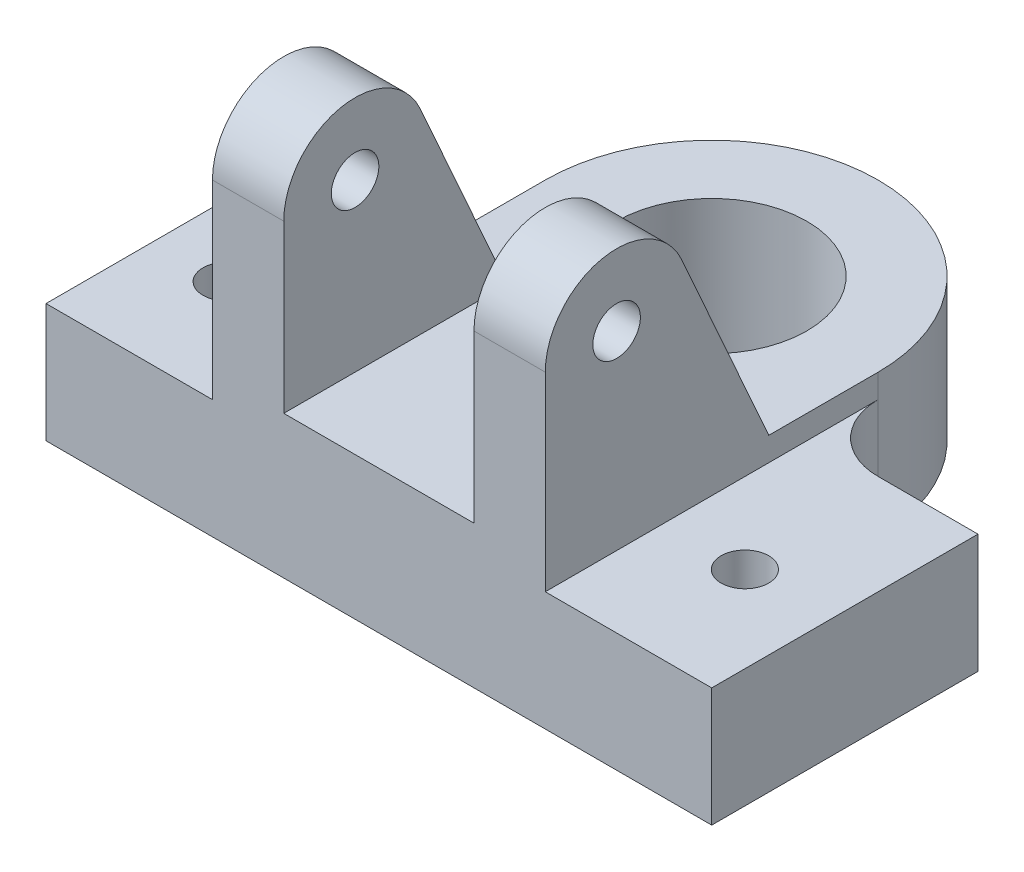
ISO-10303-21;
HEADER;
FILE_DESCRIPTION(('STEP AP214'),'2;1');
FILE_NAME('part.step','',(''),(''),'','','');
FILE_SCHEMA(('AUTOMOTIVE_DESIGN { 1 0 10303 214 1 1 1 1 }'));
ENDSEC;
DATA;
#1=APPLICATION_CONTEXT('core data for automotive mechanical design processes');
#2=APPLICATION_PROTOCOL_DEFINITION('international standard','automotive_design',2000,#1);
#3=PRODUCT_CONTEXT('',#1,'mechanical');
#4=PRODUCT('Part','Part','',(#3));
#5=PRODUCT_RELATED_PRODUCT_CATEGORY('part','',(#4));
#6=PRODUCT_DEFINITION_FORMATION('','',#4);
#7=PRODUCT_DEFINITION_CONTEXT('part definition',#1,'design');
#8=PRODUCT_DEFINITION('design','',#6,#7);
#9=PRODUCT_DEFINITION_SHAPE('','',#8);
#10=(LENGTH_UNIT() NAMED_UNIT(*) SI_UNIT(.MILLI.,.METRE.));
#11=(NAMED_UNIT(*) PLANE_ANGLE_UNIT() SI_UNIT($,.RADIAN.));
#12=(NAMED_UNIT(*) SI_UNIT($,.STERADIAN.) SOLID_ANGLE_UNIT());
#13=UNCERTAINTY_MEASURE_WITH_UNIT(LENGTH_MEASURE(1.E-05),#10,'distance_accuracy_value','');
#14=(GEOMETRIC_REPRESENTATION_CONTEXT(3) GLOBAL_UNCERTAINTY_ASSIGNED_CONTEXT((#13)) GLOBAL_UNIT_ASSIGNED_CONTEXT((#10,
#11,#12)) REPRESENTATION_CONTEXT('',''));
#15=CARTESIAN_POINT('',(0.,0.,0.));
#16=DIRECTION('',(0.,0.,1.));
#17=DIRECTION('',(1.,0.,0.));
#18=AXIS2_PLACEMENT_3D('',#15,#16,#17);
#19=CARTESIAN_POINT('',(-70.,25.,31.7302464178724));
#20=DIRECTION('',(0.,0.,-1.));
#21=DIRECTION('',(-1.,0.,0.));
#22=AXIS2_PLACEMENT_3D('',#19,#20,#21);
#23=PLANE('',#22);
#24=DIRECTION('',(0.,-1.,0.));
#25=VECTOR('',#24,1.);
#26=CARTESIAN_POINT('',(-20.,237.,31.7302464178724));
#27=LINE('',#26,#25);
#28=CARTESIAN_POINT('',(-20.,65.0000000000001,31.7302464178724));
#29=VERTEX_POINT('',#28);
#30=CARTESIAN_POINT('',(-20.,30.,31.7302464178724));
#31=VERTEX_POINT('',#30);
#32=EDGE_CURVE('E167',#29,#31,#27,.T.);
#33=ORIENTED_EDGE('',*,*,#32,.F.);
#34=DIRECTION('',(1.,0.,0.));
#35=VECTOR('',#34,1.);
#36=CARTESIAN_POINT('',(-35.,65.,31.7302464178724));
#37=LINE('',#36,#35);
#38=CARTESIAN_POINT('',(-35.,65.,31.7302464178724));
#39=VERTEX_POINT('',#38);
#40=EDGE_CURVE('E192',#39,#29,#37,.T.);
#41=ORIENTED_EDGE('',*,*,#40,.F.);
#42=DIRECTION('',(0.,-1.,0.));
#43=VECTOR('',#42,1.);
#44=CARTESIAN_POINT('',(-35.,30.,31.7302464178724));
#45=LINE('',#44,#43);
#46=CARTESIAN_POINT('',(-35.,25.,31.7302464178724));
#47=VERTEX_POINT('',#46);
#48=EDGE_CURVE('E235',#39,#47,#45,.T.);
#49=ORIENTED_EDGE('',*,*,#48,.T.);
#50=DIRECTION('',(1.,0.,0.));
#51=VECTOR('',#50,1.);
#52=CARTESIAN_POINT('',(-70.,25.,31.7302464178724));
#53=LINE('',#52,#51);
#54=CARTESIAN_POINT('',(-70.,25.,31.7302464178724));
#55=VERTEX_POINT('',#54);
#56=EDGE_CURVE('E274',#55,#47,#53,.T.);
#57=ORIENTED_EDGE('',*,*,#56,.F.);
#58=DIRECTION('',(0.,-1.,0.));
#59=VECTOR('',#58,1.);
#60=CARTESIAN_POINT('',(-70.,25.,31.7302464178724));
#61=LINE('',#60,#59);
#62=CARTESIAN_POINT('',(-70.,0.,31.7302464178724));
#63=VERTEX_POINT('',#62);
#64=EDGE_CURVE('E283',#55,#63,#61,.T.);
#65=ORIENTED_EDGE('',*,*,#64,.T.);
#66=DIRECTION('',(1.,0.,0.));
#67=VECTOR('',#66,1.);
#68=CARTESIAN_POINT('',(-70.,0.,31.7302464178724));
#69=LINE('',#68,#67);
#70=CARTESIAN_POINT('',(70.,0.,31.7302464178724));
#71=VERTEX_POINT('',#70);
#72=EDGE_CURVE('E280',#63,#71,#69,.T.);
#73=ORIENTED_EDGE('',*,*,#72,.T.);
#74=DIRECTION('',(0.,-1.,0.));
#75=VECTOR('',#74,1.);
#76=CARTESIAN_POINT('',(70.,25.,31.7302464178724));
#77=LINE('',#76,#75);
#78=CARTESIAN_POINT('',(70.,25.,31.7302464178724));
#79=VERTEX_POINT('',#78);
#80=EDGE_CURVE('E279',#79,#71,#77,.T.);
#81=ORIENTED_EDGE('',*,*,#80,.F.);
#82=CARTESIAN_POINT('',(35.,25.,31.7302464178724));
#83=VERTEX_POINT('',#82);
#84=EDGE_CURVE('E271',#83,#79,#53,.T.);
#85=ORIENTED_EDGE('',*,*,#84,.F.);
#86=DIRECTION('',(0.,-1.,0.));
#87=VECTOR('',#86,1.);
#88=CARTESIAN_POINT('',(35.,30.,31.7302464178724));
#89=LINE('',#88,#87);
#90=CARTESIAN_POINT('',(35.,65.,31.7302464178724));
#91=VERTEX_POINT('',#90);
#92=EDGE_CURVE('E230',#91,#83,#89,.T.);
#93=ORIENTED_EDGE('',*,*,#92,.F.);
#94=CARTESIAN_POINT('',(20.,65.,31.7302464178724));
#95=VERTEX_POINT('',#94);
#96=EDGE_CURVE('E204',#95,#91,#37,.T.);
#97=ORIENTED_EDGE('',*,*,#96,.F.);
#98=DIRECTION('',(0.,-1.,0.));
#99=VECTOR('',#98,1.);
#100=CARTESIAN_POINT('',(20.,237.,31.7302464178725));
#101=LINE('',#100,#99);
#102=CARTESIAN_POINT('',(20.,30.,31.7302464178725));
#103=VERTEX_POINT('',#102);
#104=EDGE_CURVE('E56',#95,#103,#101,.T.);
#105=ORIENTED_EDGE('',*,*,#104,.T.);
#106=DIRECTION('',(1.,0.,0.));
#107=VECTOR('',#106,1.);
#108=CARTESIAN_POINT('',(-20.,30.,31.7302464178724));
#109=LINE('',#108,#107);
#110=EDGE_CURVE('E173',#31,#103,#109,.T.);
#111=ORIENTED_EDGE('',*,*,#110,.F.);
#112=EDGE_LOOP('',(#33,#41,#49,#57,#65,#73,#81,#85,#93,#97,#105,#111));
#113=FACE_BOUND('',#112,.T.);
#114=ADVANCED_FACE('F43',(#113),#23,.F.);
#115=CARTESIAN_POINT('',(-35.,10.635177862415,-23.8903273022607));
#116=DIRECTION('',(0.,0.406689373293844,-0.913566502040142));
#117=DIRECTION('',(0.,0.913566502040142,0.406689373293844));
#118=AXIS2_PLACEMENT_3D('',#115,#116,#117);
#119=PLANE('',#118);
#120=DIRECTION('',(1.,0.,0.));
#121=VECTOR('',#120,1.);
#122=CARTESIAN_POINT('',(-35.,71.1003405994077,3.02674888727032));
#123=LINE('',#122,#121);
#124=CARTESIAN_POINT('',(-35.,71.1003405994077,3.02674888727032));
#125=VERTEX_POINT('',#124);
#126=CARTESIAN_POINT('',(-20.,71.1003405994077,3.02674888727032));
#127=VERTEX_POINT('',#126);
#128=EDGE_CURVE('E185',#125,#127,#123,.T.);
#129=ORIENTED_EDGE('',*,*,#128,.T.);
#130=DIRECTION('',(0.,-0.913566502040142,-0.406689373293844));
#131=VECTOR('',#130,1.);
#132=CARTESIAN_POINT('',(-20.,10.635177862415,-23.8903273022607));
#133=LINE('',#132,#131);
#134=CARTESIAN_POINT('',(-20.,30.,-15.2697535821276));
#135=VERTEX_POINT('',#134);
#136=EDGE_CURVE('E166',#127,#135,#133,.T.);
#137=ORIENTED_EDGE('',*,*,#136,.T.);
#138=DIRECTION('',(1.,0.,0.));
#139=VECTOR('',#138,1.);
#140=CARTESIAN_POINT('',(-35.,30.,-15.2697535821276));
#141=LINE('',#140,#139);
#142=CARTESIAN_POINT('',(-35.,30.,-15.2697535821276));
#143=VERTEX_POINT('',#142);
#144=EDGE_CURVE('E179',#143,#135,#141,.T.);
#145=ORIENTED_EDGE('',*,*,#144,.F.);
#146=DIRECTION('',(0.,0.913566502040142,0.406689373293844));
#147=VECTOR('',#146,1.);
#148=CARTESIAN_POINT('',(-35.,10.635177862415,-23.8903273022607));
#149=LINE('',#148,#147);
#150=EDGE_CURVE('E319',#143,#125,#149,.T.);
#151=ORIENTED_EDGE('',*,*,#150,.T.);
#152=EDGE_LOOP('',(#129,#137,#145,#151));
#153=FACE_BOUND('',#152,.T.);
#154=ADVANCED_FACE('F178',(#153),#119,.T.);
#155=CARTESIAN_POINT('',(20.,30.,-15.2697535821276));
#156=VERTEX_POINT('',#155);
#157=CARTESIAN_POINT('',(35.,30.,-15.2697535821276));
#158=VERTEX_POINT('',#157);
#159=EDGE_CURVE('E66',#156,#158,#141,.T.);
#160=ORIENTED_EDGE('',*,*,#159,.F.);
#161=DIRECTION('',(0.,0.913566502040142,0.406689373293844));
#162=VECTOR('',#161,1.);
#163=CARTESIAN_POINT('',(20.,10.635177862415,-23.8903273022607));
#164=LINE('',#163,#162);
#165=CARTESIAN_POINT('',(20.,71.1003405994077,3.02674888727032));
#166=VERTEX_POINT('',#165);
#167=EDGE_CURVE('E183',#156,#166,#164,.T.);
#168=ORIENTED_EDGE('',*,*,#167,.T.);
#169=CARTESIAN_POINT('',(35.,71.1003405994077,3.02674888727032));
#170=VERTEX_POINT('',#169);
#171=EDGE_CURVE('E205',#166,#170,#123,.T.);
#172=ORIENTED_EDGE('',*,*,#171,.T.);
#173=DIRECTION('',(0.,0.913566502040142,0.406689373293844));
#174=VECTOR('',#173,1.);
#175=CARTESIAN_POINT('',(35.,10.635177862415,-23.8903273022607));
#176=LINE('',#175,#174);
#177=EDGE_CURVE('E182',#158,#170,#176,.T.);
#178=ORIENTED_EDGE('',*,*,#177,.F.);
#179=EDGE_LOOP('',(#160,#168,#172,#178));
#180=FACE_BOUND('',#179,.T.);
#181=ADVANCED_FACE('F363',(#180),#119,.T.);
#182=CARTESIAN_POINT('',(-35.,65.,16.7302464178725));
#183=DIRECTION('',(1.,0.,0.));
#184=DIRECTION('',(0.,0.,-1.));
#185=AXIS2_PLACEMENT_3D('',#182,#183,#184);
#186=CYLINDRICAL_SURFACE('',#185,15.);
#187=ORIENTED_EDGE('',*,*,#40,.T.);
#188=CARTESIAN_POINT('',(-20.,65.,16.7302464178725));
#189=DIRECTION('',(1.,0.,0.));
#190=DIRECTION('',(0.,0.,-1.));
#191=AXIS2_PLACEMENT_3D('',#188,#189,#190);
#192=CIRCLE('',#191,15.);
#193=EDGE_CURVE('E11',#29,#127,#192,.F.);
#194=ORIENTED_EDGE('',*,*,#193,.T.);
#195=ORIENTED_EDGE('',*,*,#128,.F.);
#196=CARTESIAN_POINT('',(-35.,65.,16.7302464178725));
#197=DIRECTION('',(1.,0.,0.));
#198=DIRECTION('',(0.,0.,-1.));
#199=AXIS2_PLACEMENT_3D('',#196,#197,#198);
#200=CIRCLE('',#199,15.);
#201=EDGE_CURVE('E316',#125,#39,#200,.T.);
#202=ORIENTED_EDGE('',*,*,#201,.T.);
#203=EDGE_LOOP('',(#187,#194,#195,#202));
#204=FACE_BOUND('',#203,.T.);
#205=ADVANCED_FACE('F417',(#204),#186,.T.);
#206=ORIENTED_EDGE('',*,*,#171,.F.);
#207=CARTESIAN_POINT('',(20.,65.,16.7302464178725));
#208=DIRECTION('',(-1.,0.,0.));
#209=DIRECTION('',(0.,0.,1.));
#210=AXIS2_PLACEMENT_3D('',#207,#208,#209);
#211=CIRCLE('',#210,15.);
#212=EDGE_CURVE('E55',#166,#95,#211,.F.);
#213=ORIENTED_EDGE('',*,*,#212,.T.);
#214=ORIENTED_EDGE('',*,*,#96,.T.);
#215=CARTESIAN_POINT('',(35.,65.,16.7302464178725));
#216=DIRECTION('',(1.,0.,0.));
#217=DIRECTION('',(0.,0.,-1.));
#218=AXIS2_PLACEMENT_3D('',#215,#216,#217);
#219=CIRCLE('',#218,15.);
#220=EDGE_CURVE('E200',#170,#91,#219,.T.);
#221=ORIENTED_EDGE('',*,*,#220,.F.);
#222=EDGE_LOOP('',(#206,#213,#214,#221));
#223=FACE_BOUND('',#222,.T.);
#224=ADVANCED_FACE('F306',(#223),#186,.T.);
#225=CARTESIAN_POINT('',(0.,30.,0.));
#226=DIRECTION('',(0.,1.,0.));
#227=DIRECTION('',(0.,0.,1.));
#228=AXIS2_PLACEMENT_3D('',#225,#226,#227);
#229=PLANE('',#228);
#230=CARTESIAN_POINT('',(0.,30.,-38.2697535821276));
#231=DIRECTION('',(0.,1.,0.));
#232=DIRECTION('',(0.,0.,1.));
#233=AXIS2_PLACEMENT_3D('',#230,#231,#232);
#234=CIRCLE('',#233,20.);
#235=CARTESIAN_POINT('',(0.,30.,-18.2697535821276));
#236=VERTEX_POINT('',#235);
#237=EDGE_CURVE('E212',#236,#236,#234,.F.);
#238=ORIENTED_EDGE('',*,*,#237,.T.);
#239=EDGE_LOOP('',(#238));
#240=FACE_BOUND('',#239,.T.);
#241=DIRECTION('',(0.,0.,1.));
#242=VECTOR('',#241,1.);
#243=CARTESIAN_POINT('',(-35.,30.,0.));
#244=LINE('',#243,#242);
#245=CARTESIAN_POINT('',(-35.,30.,-38.2697535821276));
#246=VERTEX_POINT('',#245);
#247=EDGE_CURVE('E186',#246,#143,#244,.T.);
#248=ORIENTED_EDGE('',*,*,#247,.T.);
#249=ORIENTED_EDGE('',*,*,#144,.T.);
#250=DIRECTION('',(0.,0.,1.));
#251=VECTOR('',#250,1.);
#252=CARTESIAN_POINT('',(-20.,30.,-15.2697535821276));
#253=LINE('',#252,#251);
#254=EDGE_CURVE('E164',#135,#31,#253,.T.);
#255=ORIENTED_EDGE('',*,*,#254,.T.);
#256=ORIENTED_EDGE('',*,*,#110,.T.);
#257=DIRECTION('',(0.,0.,-1.));
#258=VECTOR('',#257,1.);
#259=CARTESIAN_POINT('',(20.,30.,-15.2697535821276));
#260=LINE('',#259,#258);
#261=EDGE_CURVE('E326',#103,#156,#260,.T.);
#262=ORIENTED_EDGE('',*,*,#261,.T.);
#263=ORIENTED_EDGE('',*,*,#159,.T.);
#264=DIRECTION('',(0.,0.,1.));
#265=VECTOR('',#264,1.);
#266=CARTESIAN_POINT('',(35.,30.,0.));
#267=LINE('',#266,#265);
#268=CARTESIAN_POINT('',(35.,30.,-38.2697535821275));
#269=VERTEX_POINT('',#268);
#270=EDGE_CURVE('E217',#269,#158,#267,.T.);
#271=ORIENTED_EDGE('',*,*,#270,.F.);
#272=CARTESIAN_POINT('',(0.,30.,-38.2697535821276));
#273=DIRECTION('',(0.,1.,0.));
#274=DIRECTION('',(0.,0.,1.));
#275=AXIS2_PLACEMENT_3D('',#272,#273,#274);
#276=CIRCLE('',#275,35.);
#277=EDGE_CURVE('E219',#269,#246,#276,.T.);
#278=ORIENTED_EDGE('',*,*,#277,.T.);
#279=EDGE_LOOP('',(#248,#249,#255,#256,#262,#263,#271,#278));
#280=FACE_BOUND('',#279,.T.);
#281=ADVANCED_FACE('F190',(#240,#280),#229,.T.);
#282=CARTESIAN_POINT('',(0.,25.,0.));
#283=DIRECTION('',(0.,-1.,0.));
#284=DIRECTION('',(0.,0.,-1.));
#285=AXIS2_PLACEMENT_3D('',#282,#283,#284);
#286=PLANE('',#285);
#287=CARTESIAN_POINT('',(-55.,25.,8.73024641787245));
#288=DIRECTION('',(0.,1.,0.));
#289=DIRECTION('',(0.,0.,1.));
#290=AXIS2_PLACEMENT_3D('',#287,#288,#289);
#291=CIRCLE('',#290,5.);
#292=CARTESIAN_POINT('',(-55.,25.,13.7302464178724));
#293=VERTEX_POINT('',#292);
#294=EDGE_CURVE('E210',#293,#293,#291,.T.);
#295=ORIENTED_EDGE('',*,*,#294,.F.);
#296=EDGE_LOOP('',(#295));
#297=FACE_BOUND('',#296,.T.);
#298=DIRECTION('',(0.,0.,1.));
#299=VECTOR('',#298,1.);
#300=CARTESIAN_POINT('',(-35.,25.,0.));
#301=LINE('',#300,#299);
#302=CARTESIAN_POINT('',(-35.,25.,-38.2697535821276));
#303=VERTEX_POINT('',#302);
#304=EDGE_CURVE('E213',#303,#47,#301,.T.);
#305=ORIENTED_EDGE('',*,*,#304,.F.);
#306=CARTESIAN_POINT('',(-49.,25.,-38.2697535821275));
#307=DIRECTION('',(0.,-1.,0.));
#308=DIRECTION('',(0.,0.,-1.));
#309=AXIS2_PLACEMENT_3D('',#306,#307,#308);
#310=CIRCLE('',#309,14.);
#311=CARTESIAN_POINT('',(-49.,25.,-24.2697535821276));
#312=VERTEX_POINT('',#311);
#313=EDGE_CURVE('E257',#312,#303,#310,.F.);
#314=ORIENTED_EDGE('',*,*,#313,.F.);
#315=DIRECTION('',(-1.,0.,0.));
#316=VECTOR('',#315,1.);
#317=CARTESIAN_POINT('',(0.,25.,-24.2697535821275));
#318=LINE('',#317,#316);
#319=CARTESIAN_POINT('',(-70.,25.,-24.2697535821276));
#320=VERTEX_POINT('',#319);
#321=EDGE_CURVE('E265',#312,#320,#318,.T.);
#322=ORIENTED_EDGE('',*,*,#321,.T.);
#323=DIRECTION('',(0.,0.,1.));
#324=VECTOR('',#323,1.);
#325=CARTESIAN_POINT('',(-70.,25.,-73.2697535821275));
#326=LINE('',#325,#324);
#327=EDGE_CURVE('E266',#320,#55,#326,.T.);
#328=ORIENTED_EDGE('',*,*,#327,.T.);
#329=ORIENTED_EDGE('',*,*,#56,.T.);
#330=EDGE_LOOP('',(#305,#314,#322,#328,#329));
#331=FACE_BOUND('',#330,.T.);
#332=ADVANCED_FACE('F380',(#297,#331),#286,.F.);
#333=CARTESIAN_POINT('',(-70.,25.,-73.2697535821275));
#334=DIRECTION('',(1.,0.,0.));
#335=DIRECTION('',(0.,0.,-1.));
#336=AXIS2_PLACEMENT_3D('',#333,#334,#335);
#337=PLANE('',#336);
#338=ORIENTED_EDGE('',*,*,#327,.F.);
#339=DIRECTION('',(0.,-1.,0.));
#340=VECTOR('',#339,1.);
#341=CARTESIAN_POINT('',(-70.,86.,-24.2697535821276));
#342=LINE('',#341,#340);
#343=CARTESIAN_POINT('',(-70.,0.,-24.2697535821276));
#344=VERTEX_POINT('',#343);
#345=EDGE_CURVE('E238',#320,#344,#342,.T.);
#346=ORIENTED_EDGE('',*,*,#345,.T.);
#347=DIRECTION('',(0.,0.,1.));
#348=VECTOR('',#347,1.);
#349=CARTESIAN_POINT('',(-70.,0.,-73.2697535821275));
#350=LINE('',#349,#348);
#351=EDGE_CURVE('E268',#344,#63,#350,.T.);
#352=ORIENTED_EDGE('',*,*,#351,.T.);
#353=ORIENTED_EDGE('',*,*,#64,.F.);
#354=EDGE_LOOP('',(#338,#346,#352,#353));
#355=FACE_BOUND('',#354,.T.);
#356=ADVANCED_FACE('F44',(#355),#337,.F.);
#357=CARTESIAN_POINT('',(70.,25.,-73.2697535821275));
#358=DIRECTION('',(-1.,0.,0.));
#359=DIRECTION('',(0.,0.,1.));
#360=AXIS2_PLACEMENT_3D('',#357,#358,#359);
#361=PLANE('',#360);
#362=DIRECTION('',(0.,0.,-1.));
#363=VECTOR('',#362,1.);
#364=CARTESIAN_POINT('',(70.,0.,-73.2697535821275));
#365=LINE('',#364,#363);
#366=CARTESIAN_POINT('',(70.,0.,-24.2697535821276));
#367=VERTEX_POINT('',#366);
#368=EDGE_CURVE('E272',#71,#367,#365,.T.);
#369=ORIENTED_EDGE('',*,*,#368,.T.);
#370=DIRECTION('',(0.,-1.,0.));
#371=VECTOR('',#370,1.);
#372=CARTESIAN_POINT('',(70.,86.,-24.2697535821276));
#373=LINE('',#372,#371);
#374=CARTESIAN_POINT('',(70.,25.,-24.2697535821276));
#375=VERTEX_POINT('',#374);
#376=EDGE_CURVE('E241',#375,#367,#373,.T.);
#377=ORIENTED_EDGE('',*,*,#376,.F.);
#378=DIRECTION('',(0.,0.,-1.));
#379=VECTOR('',#378,1.);
#380=CARTESIAN_POINT('',(70.,25.,-73.2697535821275));
#381=LINE('',#380,#379);
#382=EDGE_CURVE('E269',#79,#375,#381,.T.);
#383=ORIENTED_EDGE('',*,*,#382,.F.);
#384=ORIENTED_EDGE('',*,*,#80,.T.);
#385=EDGE_LOOP('',(#369,#377,#383,#384));
#386=FACE_BOUND('',#385,.T.);
#387=ADVANCED_FACE('F364',(#386),#361,.F.);
#388=CARTESIAN_POINT('',(51.91396765625,25.,6.66646532412255));
#389=DIRECTION('',(0.,-1.,0.));
#390=DIRECTION('',(0.,0.,-1.));
#391=AXIS2_PLACEMENT_3D('',#388,#389,#390);
#392=CIRCLE('',#391,5.);
#393=CARTESIAN_POINT('',(51.91396765625,25.,1.66646532412255));
#394=VERTEX_POINT('',#393);
#395=EDGE_CURVE('E195',#394,#394,#392,.F.);
#396=ORIENTED_EDGE('',*,*,#395,.F.);
#397=EDGE_LOOP('',(#396));
#398=FACE_BOUND('',#397,.T.);
#399=CARTESIAN_POINT('',(49.,25.,-38.2697535821275));
#400=DIRECTION('',(0.,-1.,0.));
#401=DIRECTION('',(0.,0.,-1.));
#402=AXIS2_PLACEMENT_3D('',#399,#400,#401);
#403=CIRCLE('',#402,14.);
#404=CARTESIAN_POINT('',(35.,25.,-38.2697535821275));
#405=VERTEX_POINT('',#404);
#406=CARTESIAN_POINT('',(49.,25.,-24.2697535821276));
#407=VERTEX_POINT('',#406);
#408=EDGE_CURVE('E260',#405,#407,#403,.F.);
#409=ORIENTED_EDGE('',*,*,#408,.F.);
#410=DIRECTION('',(0.,0.,1.));
#411=VECTOR('',#410,1.);
#412=CARTESIAN_POINT('',(35.,25.,0.));
#413=LINE('',#412,#411);
#414=EDGE_CURVE('E220',#405,#83,#413,.T.);
#415=ORIENTED_EDGE('',*,*,#414,.T.);
#416=ORIENTED_EDGE('',*,*,#84,.T.);
#417=ORIENTED_EDGE('',*,*,#382,.T.);
#418=DIRECTION('',(-1.,0.,0.));
#419=VECTOR('',#418,1.);
#420=CARTESIAN_POINT('',(0.,25.,-24.2697535821276));
#421=LINE('',#420,#419);
#422=EDGE_CURVE('E253',#375,#407,#421,.T.);
#423=ORIENTED_EDGE('',*,*,#422,.T.);
#424=EDGE_LOOP('',(#409,#415,#416,#417,#423));
#425=FACE_BOUND('',#424,.T.);
#426=ADVANCED_FACE('F370',(#398,#425),#286,.F.);
#427=CARTESIAN_POINT('',(0.,0.,0.));
#428=DIRECTION('',(0.,-1.,0.));
#429=DIRECTION('',(0.,0.,-1.));
#430=AXIS2_PLACEMENT_3D('',#427,#428,#429);
#431=PLANE('',#430);
#432=CARTESIAN_POINT('',(51.91396765625,0.,6.66646532412255));
#433=DIRECTION('',(0.,-1.,0.));
#434=DIRECTION('',(0.,0.,-1.));
#435=AXIS2_PLACEMENT_3D('',#432,#433,#434);
#436=CIRCLE('',#435,5.);
#437=CARTESIAN_POINT('',(51.91396765625,0.,1.66646532412255));
#438=VERTEX_POINT('',#437);
#439=EDGE_CURVE('E188',#438,#438,#436,.F.);
#440=ORIENTED_EDGE('',*,*,#439,.T.);
#441=EDGE_LOOP('',(#440));
#442=FACE_BOUND('',#441,.T.);
#443=CARTESIAN_POINT('',(-55.,0.,8.73024641787245));
#444=DIRECTION('',(0.,-1.,0.));
#445=DIRECTION('',(0.,0.,-1.));
#446=AXIS2_PLACEMENT_3D('',#443,#444,#445);
#447=CIRCLE('',#446,5.);
#448=CARTESIAN_POINT('',(-55.,0.,3.73024641787245));
#449=VERTEX_POINT('',#448);
#450=EDGE_CURVE('E208',#449,#449,#447,.T.);
#451=ORIENTED_EDGE('',*,*,#450,.F.);
#452=EDGE_LOOP('',(#451));
#453=FACE_BOUND('',#452,.T.);
#454=CARTESIAN_POINT('',(0.,0.,-38.2697535821276));
#455=DIRECTION('',(0.,-1.,0.));
#456=DIRECTION('',(0.,0.,-1.));
#457=AXIS2_PLACEMENT_3D('',#454,#455,#456);
#458=CIRCLE('',#457,20.);
#459=CARTESIAN_POINT('',(0.,0.,-58.2697535821276));
#460=VERTEX_POINT('',#459);
#461=EDGE_CURVE('E214',#460,#460,#458,.F.);
#462=ORIENTED_EDGE('',*,*,#461,.T.);
#463=EDGE_LOOP('',(#462));
#464=FACE_BOUND('',#463,.T.);
#465=DIRECTION('',(-1.,0.,0.));
#466=VECTOR('',#465,1.);
#467=CARTESIAN_POINT('',(0.,0.,-24.2697535821275));
#468=LINE('',#467,#466);
#469=CARTESIAN_POINT('',(-49.,0.,-24.2697535821276));
#470=VERTEX_POINT('',#469);
#471=EDGE_CURVE('E300',#470,#344,#468,.T.);
#472=ORIENTED_EDGE('',*,*,#471,.F.);
#473=CARTESIAN_POINT('',(-49.,0.,-38.2697535821275));
#474=DIRECTION('',(0.,-1.,0.));
#475=DIRECTION('',(0.,0.,-1.));
#476=AXIS2_PLACEMENT_3D('',#473,#474,#475);
#477=CIRCLE('',#476,14.);
#478=CARTESIAN_POINT('',(-35.,0.,-38.2697535821276));
#479=VERTEX_POINT('',#478);
#480=EDGE_CURVE('E295',#470,#479,#477,.F.);
#481=ORIENTED_EDGE('',*,*,#480,.T.);
#482=CARTESIAN_POINT('',(0.,0.,-38.2697535821276));
#483=DIRECTION('',(0.,-1.,0.));
#484=DIRECTION('',(0.,0.,-1.));
#485=AXIS2_PLACEMENT_3D('',#482,#483,#484);
#486=CIRCLE('',#485,35.);
#487=CARTESIAN_POINT('',(35.,0.,-38.2697535821275));
#488=VERTEX_POINT('',#487);
#489=EDGE_CURVE('E292',#488,#479,#486,.F.);
#490=ORIENTED_EDGE('',*,*,#489,.F.);
#491=CARTESIAN_POINT('',(49.,0.,-38.2697535821275));
#492=DIRECTION('',(0.,-1.,0.));
#493=DIRECTION('',(0.,0.,-1.));
#494=AXIS2_PLACEMENT_3D('',#491,#492,#493);
#495=CIRCLE('',#494,14.);
#496=CARTESIAN_POINT('',(49.,0.,-24.2697535821276));
#497=VERTEX_POINT('',#496);
#498=EDGE_CURVE('E290',#488,#497,#495,.F.);
#499=ORIENTED_EDGE('',*,*,#498,.T.);
#500=DIRECTION('',(-1.,0.,0.));
#501=VECTOR('',#500,1.);
#502=CARTESIAN_POINT('',(0.,0.,-24.2697535821276));
#503=LINE('',#502,#501);
#504=EDGE_CURVE('E289',#367,#497,#503,.T.);
#505=ORIENTED_EDGE('',*,*,#504,.F.);
#506=ORIENTED_EDGE('',*,*,#368,.F.);
#507=ORIENTED_EDGE('',*,*,#72,.F.);
#508=ORIENTED_EDGE('',*,*,#351,.F.);
#509=EDGE_LOOP('',(#472,#481,#490,#499,#505,#506,#507,#508));
#510=FACE_BOUND('',#509,.T.);
#511=ADVANCED_FACE('F367',(#442,#453,#464,#510),#431,.T.);
#512=CARTESIAN_POINT('',(0.,86.,-24.2697535821275));
#513=DIRECTION('',(0.,0.,1.));
#514=DIRECTION('',(1.,0.,0.));
#515=AXIS2_PLACEMENT_3D('',#512,#513,#514);
#516=PLANE('',#515);
#517=DIRECTION('',(0.,-1.,0.));
#518=VECTOR('',#517,1.);
#519=CARTESIAN_POINT('',(-49.,86.,-24.2697535821276));
#520=LINE('',#519,#518);
#521=EDGE_CURVE('E255',#312,#470,#520,.T.);
#522=ORIENTED_EDGE('',*,*,#521,.T.);
#523=ORIENTED_EDGE('',*,*,#471,.T.);
#524=ORIENTED_EDGE('',*,*,#345,.F.);
#525=ORIENTED_EDGE('',*,*,#321,.F.);
#526=EDGE_LOOP('',(#522,#523,#524,#525));
#527=FACE_BOUND('',#526,.T.);
#528=ADVANCED_FACE('F375',(#527),#516,.F.);
#529=CARTESIAN_POINT('',(-49.,86.,-38.2697535821275));
#530=DIRECTION('',(0.,-1.,0.));
#531=DIRECTION('',(0.,0.,-1.));
#532=AXIS2_PLACEMENT_3D('',#529,#530,#531);
#533=CYLINDRICAL_SURFACE('',#532,14.);
#534=ORIENTED_EDGE('',*,*,#313,.T.);
#535=DIRECTION('',(0.,-1.,0.));
#536=VECTOR('',#535,1.);
#537=CARTESIAN_POINT('',(-35.,86.,-38.2697535821276));
#538=LINE('',#537,#536);
#539=EDGE_CURVE('E248',#303,#479,#538,.T.);
#540=ORIENTED_EDGE('',*,*,#539,.T.);
#541=ORIENTED_EDGE('',*,*,#480,.F.);
#542=ORIENTED_EDGE('',*,*,#521,.F.);
#543=EDGE_LOOP('',(#534,#540,#541,#542));
#544=FACE_BOUND('',#543,.T.);
#545=ADVANCED_FACE('F379',(#544),#533,.F.);
#546=CARTESIAN_POINT('',(0.,86.,-38.2697535821276));
#547=DIRECTION('',(0.,-1.,0.));
#548=DIRECTION('',(0.,0.,-1.));
#549=AXIS2_PLACEMENT_3D('',#546,#547,#548);
#550=CYLINDRICAL_SURFACE('',#549,35.);
#551=DIRECTION('',(0.,-1.,0.));
#552=VECTOR('',#551,1.);
#553=CARTESIAN_POINT('',(35.,86.,-38.2697535821275));
#554=LINE('',#553,#552);
#555=EDGE_CURVE('E246',#405,#488,#554,.T.);
#556=ORIENTED_EDGE('',*,*,#555,.T.);
#557=ORIENTED_EDGE('',*,*,#489,.T.);
#558=ORIENTED_EDGE('',*,*,#539,.F.);
#559=DIRECTION('',(0.,-1.,0.));
#560=VECTOR('',#559,1.);
#561=CARTESIAN_POINT('',(-35.,30.,-38.2697535821276));
#562=LINE('',#561,#560);
#563=EDGE_CURVE('E232',#246,#303,#562,.T.);
#564=ORIENTED_EDGE('',*,*,#563,.F.);
#565=ORIENTED_EDGE('',*,*,#277,.F.);
#566=DIRECTION('',(0.,-1.,0.));
#567=VECTOR('',#566,1.);
#568=CARTESIAN_POINT('',(35.,30.,-38.2697535821275));
#569=LINE('',#568,#567);
#570=EDGE_CURVE('E222',#269,#405,#569,.T.);
#571=ORIENTED_EDGE('',*,*,#570,.T.);
#572=EDGE_LOOP('',(#556,#557,#558,#564,#565,#571));
#573=FACE_BOUND('',#572,.T.);
#574=ADVANCED_FACE('F381',(#573),#550,.T.);
#575=CARTESIAN_POINT('',(49.,86.,-38.2697535821275));
#576=DIRECTION('',(0.,-1.,0.));
#577=DIRECTION('',(0.,0.,-1.));
#578=AXIS2_PLACEMENT_3D('',#575,#576,#577);
#579=CYLINDRICAL_SURFACE('',#578,14.);
#580=ORIENTED_EDGE('',*,*,#408,.T.);
#581=DIRECTION('',(0.,-1.,0.));
#582=VECTOR('',#581,1.);
#583=CARTESIAN_POINT('',(49.,86.,-24.2697535821276));
#584=LINE('',#583,#582);
#585=EDGE_CURVE('E243',#407,#497,#584,.T.);
#586=ORIENTED_EDGE('',*,*,#585,.T.);
#587=ORIENTED_EDGE('',*,*,#498,.F.);
#588=ORIENTED_EDGE('',*,*,#555,.F.);
#589=EDGE_LOOP('',(#580,#586,#587,#588));
#590=FACE_BOUND('',#589,.T.);
#591=ADVANCED_FACE('F390',(#590),#579,.F.);
#592=CARTESIAN_POINT('',(0.,86.,-24.2697535821276));
#593=DIRECTION('',(0.,0.,1.));
#594=DIRECTION('',(1.,0.,0.));
#595=AXIS2_PLACEMENT_3D('',#592,#593,#594);
#596=PLANE('',#595);
#597=ORIENTED_EDGE('',*,*,#376,.T.);
#598=ORIENTED_EDGE('',*,*,#504,.T.);
#599=ORIENTED_EDGE('',*,*,#585,.F.);
#600=ORIENTED_EDGE('',*,*,#422,.F.);
#601=EDGE_LOOP('',(#597,#598,#599,#600));
#602=FACE_BOUND('',#601,.T.);
#603=ADVANCED_FACE('F391',(#602),#596,.F.);
#604=CARTESIAN_POINT('',(-35.,30.,0.));
#605=DIRECTION('',(1.,0.,0.));
#606=DIRECTION('',(0.,0.,-1.));
#607=AXIS2_PLACEMENT_3D('',#604,#605,#606);
#608=PLANE('',#607);
#609=CARTESIAN_POINT('',(-35.,65.,16.7302464178725));
#610=DIRECTION('',(1.,0.,0.));
#611=DIRECTION('',(0.,0.,-1.));
#612=AXIS2_PLACEMENT_3D('',#609,#610,#611);
#613=CIRCLE('',#612,5.);
#614=CARTESIAN_POINT('',(-35.,65.,11.7302464178724));
#615=VERTEX_POINT('',#614);
#616=EDGE_CURVE('E172',#615,#615,#613,.F.);
#617=ORIENTED_EDGE('',*,*,#616,.F.);
#618=EDGE_LOOP('',(#617));
#619=FACE_BOUND('',#618,.T.);
#620=ORIENTED_EDGE('',*,*,#304,.T.);
#621=ORIENTED_EDGE('',*,*,#48,.F.);
#622=ORIENTED_EDGE('',*,*,#201,.F.);
#623=ORIENTED_EDGE('',*,*,#150,.F.);
#624=ORIENTED_EDGE('',*,*,#247,.F.);
#625=ORIENTED_EDGE('',*,*,#563,.T.);
#626=EDGE_LOOP('',(#620,#621,#622,#623,#624,#625));
#627=FACE_BOUND('',#626,.T.);
#628=ADVANCED_FACE('F398',(#619,#627),#608,.F.);
#629=CARTESIAN_POINT('',(35.,30.,0.));
#630=DIRECTION('',(1.,0.,0.));
#631=DIRECTION('',(0.,0.,-1.));
#632=AXIS2_PLACEMENT_3D('',#629,#630,#631);
#633=PLANE('',#632);
#634=CARTESIAN_POINT('',(35.,65.,16.7302464178725));
#635=DIRECTION('',(1.,0.,0.));
#636=DIRECTION('',(0.,0.,-1.));
#637=AXIS2_PLACEMENT_3D('',#634,#635,#636);
#638=CIRCLE('',#637,5.);
#639=CARTESIAN_POINT('',(35.,65.,11.7302464178724));
#640=VERTEX_POINT('',#639);
#641=EDGE_CURVE('E334',#640,#640,#638,.F.);
#642=ORIENTED_EDGE('',*,*,#641,.T.);
#643=EDGE_LOOP('',(#642));
#644=FACE_BOUND('',#643,.T.);
#645=ORIENTED_EDGE('',*,*,#414,.F.);
#646=ORIENTED_EDGE('',*,*,#570,.F.);
#647=ORIENTED_EDGE('',*,*,#270,.T.);
#648=ORIENTED_EDGE('',*,*,#177,.T.);
#649=ORIENTED_EDGE('',*,*,#220,.T.);
#650=ORIENTED_EDGE('',*,*,#92,.T.);
#651=EDGE_LOOP('',(#645,#646,#647,#648,#649,#650));
#652=FACE_BOUND('',#651,.T.);
#653=ADVANCED_FACE('F320',(#644,#652),#633,.T.);
#654=CARTESIAN_POINT('',(0.,140.,-38.2697535821276));
#655=DIRECTION('',(0.,-1.,0.));
#656=DIRECTION('',(0.,0.,-1.));
#657=AXIS2_PLACEMENT_3D('',#654,#655,#656);
#658=CYLINDRICAL_SURFACE('',#657,20.);
#659=ORIENTED_EDGE('',*,*,#461,.F.);
#660=EDGE_LOOP('',(#659));
#661=FACE_BOUND('',#660,.T.);
#662=ORIENTED_EDGE('',*,*,#237,.F.);
#663=EDGE_LOOP('',(#662));
#664=FACE_BOUND('',#663,.T.);
#665=ADVANCED_FACE('F401',(#661,#664),#658,.F.);
#666=CARTESIAN_POINT('',(-55.,-368.,8.73024641787245));
#667=DIRECTION('',(0.,1.,0.));
#668=DIRECTION('',(0.,0.,1.));
#669=AXIS2_PLACEMENT_3D('',#666,#667,#668);
#670=CYLINDRICAL_SURFACE('',#669,5.);
#671=ORIENTED_EDGE('',*,*,#450,.T.);
#672=EDGE_LOOP('',(#671));
#673=FACE_BOUND('',#672,.T.);
#674=ORIENTED_EDGE('',*,*,#294,.T.);
#675=EDGE_LOOP('',(#674));
#676=FACE_BOUND('',#675,.T.);
#677=ADVANCED_FACE('F407',(#673,#676),#670,.F.);
#678=CARTESIAN_POINT('',(51.91396765625,418.,6.66646532412255));
#679=DIRECTION('',(0.,-1.,0.));
#680=DIRECTION('',(0.,0.,-1.));
#681=AXIS2_PLACEMENT_3D('',#678,#679,#680);
#682=CYLINDRICAL_SURFACE('',#681,5.);
#683=ORIENTED_EDGE('',*,*,#439,.F.);
#684=EDGE_LOOP('',(#683));
#685=FACE_BOUND('',#684,.T.);
#686=ORIENTED_EDGE('',*,*,#395,.T.);
#687=EDGE_LOOP('',(#686));
#688=FACE_BOUND('',#687,.T.);
#689=ADVANCED_FACE('F413',(#685,#688),#682,.F.);
#690=CARTESIAN_POINT('',(-20.,237.,-15.2697535821276));
#691=DIRECTION('',(1.,0.,0.));
#692=DIRECTION('',(0.,0.,-1.));
#693=AXIS2_PLACEMENT_3D('',#690,#691,#692);
#694=PLANE('',#693);
#695=CARTESIAN_POINT('',(-20.,65.,16.7302464178725));
#696=DIRECTION('',(1.,0.,0.));
#697=DIRECTION('',(0.,0.,-1.));
#698=AXIS2_PLACEMENT_3D('',#695,#696,#697);
#699=CIRCLE('',#698,5.);
#700=CARTESIAN_POINT('',(-20.,65.,11.7302464178724));
#701=VERTEX_POINT('',#700);
#702=EDGE_CURVE('E331',#701,#701,#699,.F.);
#703=ORIENTED_EDGE('',*,*,#702,.T.);
#704=EDGE_LOOP('',(#703));
#705=FACE_BOUND('',#704,.T.);
#706=ORIENTED_EDGE('',*,*,#193,.F.);
#707=ORIENTED_EDGE('',*,*,#32,.T.);
#708=ORIENTED_EDGE('',*,*,#254,.F.);
#709=ORIENTED_EDGE('',*,*,#136,.F.);
#710=EDGE_LOOP('',(#706,#707,#708,#709));
#711=FACE_BOUND('',#710,.T.);
#712=ADVANCED_FACE('F170',(#705,#711),#694,.T.);
#713=CARTESIAN_POINT('',(20.,237.,-15.2697535821276));
#714=DIRECTION('',(-1.,0.,0.));
#715=DIRECTION('',(0.,0.,1.));
#716=AXIS2_PLACEMENT_3D('',#713,#714,#715);
#717=PLANE('',#716);
#718=CARTESIAN_POINT('',(19.9999999999999,65.,16.7302464178725));
#719=DIRECTION('',(-1.,0.,0.));
#720=DIRECTION('',(0.,0.,1.));
#721=AXIS2_PLACEMENT_3D('',#718,#719,#720);
#722=CIRCLE('',#721,5.);
#723=CARTESIAN_POINT('',(19.9999999999999,65.,11.7302464178724));
#724=VERTEX_POINT('',#723);
#725=EDGE_CURVE('E50',#724,#724,#722,.F.);
#726=ORIENTED_EDGE('',*,*,#725,.T.);
#727=EDGE_LOOP('',(#726));
#728=FACE_BOUND('',#727,.T.);
#729=ORIENTED_EDGE('',*,*,#261,.F.);
#730=ORIENTED_EDGE('',*,*,#104,.F.);
#731=ORIENTED_EDGE('',*,*,#212,.F.);
#732=ORIENTED_EDGE('',*,*,#167,.F.);
#733=EDGE_LOOP('',(#729,#730,#731,#732));
#734=FACE_BOUND('',#733,.T.);
#735=ADVANCED_FACE('F341',(#728,#734),#717,.T.);
#736=CARTESIAN_POINT('',(-242.,65.,16.7302464178725));
#737=DIRECTION('',(1.,0.,0.));
#738=DIRECTION('',(0.,0.,-1.));
#739=AXIS2_PLACEMENT_3D('',#736,#737,#738);
#740=CYLINDRICAL_SURFACE('',#739,5.);
#741=CARTESIAN_POINT('',(35.,65.,11.7302464178724));
#742=CARTESIAN_POINT('',(34.8437499999999,65.,11.7302464178724));
#743=CARTESIAN_POINT('',(34.6874999999999,65.,11.7302464178724));
#744=CARTESIAN_POINT('',(34.3749999999999,65.,11.7302464178724));
#745=CARTESIAN_POINT('',(34.21875,65.,11.7302464178724));
#746=CARTESIAN_POINT('',(33.90625,65.,11.7302464178724));
#747=CARTESIAN_POINT('',(33.75,65.,11.7302464178724));
#748=CARTESIAN_POINT('',(33.4374999999999,65.,11.7302464178724));
#749=CARTESIAN_POINT('',(33.2812499999999,65.,11.7302464178724));
#750=CARTESIAN_POINT('',(32.9687499999999,65.,11.7302464178724));
#751=CARTESIAN_POINT('',(32.8125,65.,11.7302464178724));
#752=CARTESIAN_POINT('',(32.5,65.,11.7302464178724));
#753=CARTESIAN_POINT('',(32.34375,65.,11.7302464178724));
#754=CARTESIAN_POINT('',(32.03125,65.,11.7302464178724));
#755=CARTESIAN_POINT('',(31.8749999999999,65.,11.7302464178724));
#756=CARTESIAN_POINT('',(31.5624999999999,65.,11.7302464178724));
#757=CARTESIAN_POINT('',(31.4062499999999,65.,11.7302464178724));
#758=CARTESIAN_POINT('',(31.0937499999999,65.,11.7302464178724));
#759=CARTESIAN_POINT('',(30.9374999999999,65.,11.7302464178724));
#760=CARTESIAN_POINT('',(30.6249999999999,65.,11.7302464178724));
#761=CARTESIAN_POINT('',(30.4687499999999,65.,11.7302464178724));
#762=CARTESIAN_POINT('',(30.1562499999999,65.,11.7302464178724));
#763=CARTESIAN_POINT('',(29.9999999999999,65.,11.7302464178724));
#764=CARTESIAN_POINT('',(29.6874999999999,65.,11.7302464178724));
#765=CARTESIAN_POINT('',(29.5312499999999,65.,11.7302464178724));
#766=CARTESIAN_POINT('',(29.21875,65.,11.7302464178724));
#767=CARTESIAN_POINT('',(29.0624999999999,65.,11.7302464178724));
#768=CARTESIAN_POINT('',(28.7499999999999,65.,11.7302464178724));
#769=CARTESIAN_POINT('',(28.5937499999999,65.,11.7302464178724));
#770=CARTESIAN_POINT('',(28.2812499999999,65.,11.7302464178724));
#771=CARTESIAN_POINT('',(28.1249999999999,65.,11.7302464178724));
#772=CARTESIAN_POINT('',(27.8125,65.,11.7302464178724));
#773=CARTESIAN_POINT('',(27.6562499999999,65.,11.7302464178724));
#774=CARTESIAN_POINT('',(27.3437499999999,65.,11.7302464178724));
#775=CARTESIAN_POINT('',(27.1874999999999,65.,11.7302464178724));
#776=CARTESIAN_POINT('',(26.8749999999999,65.,11.7302464178724));
#777=CARTESIAN_POINT('',(26.7187499999999,65.,11.7302464178724));
#778=CARTESIAN_POINT('',(26.40625,65.,11.7302464178724));
#779=CARTESIAN_POINT('',(26.25,65.,11.7302464178724));
#780=CARTESIAN_POINT('',(25.9374999999999,65.,11.7302464178724));
#781=CARTESIAN_POINT('',(25.7812499999999,65.,11.7302464178724));
#782=CARTESIAN_POINT('',(25.4687499999999,65.,11.7302464178724));
#783=CARTESIAN_POINT('',(25.3125,65.,11.7302464178724));
#784=CARTESIAN_POINT('',(25.,65.,11.7302464178724));
#785=CARTESIAN_POINT('',(24.84375,65.,11.7302464178724));
#786=CARTESIAN_POINT('',(24.5312499999999,65.,11.7302464178724));
#787=CARTESIAN_POINT('',(24.3749999999999,65.,11.7302464178724));
#788=CARTESIAN_POINT('',(24.0624999999999,65.,11.7302464178724));
#789=CARTESIAN_POINT('',(23.90625,65.,11.7302464178724));
#790=CARTESIAN_POINT('',(23.59375,65.,11.7302464178724));
#791=CARTESIAN_POINT('',(23.4375,65.,11.7302464178724));
#792=CARTESIAN_POINT('',(23.1249999999999,65.,11.7302464178724));
#793=CARTESIAN_POINT('',(22.9687499999999,65.,11.7302464178724));
#794=CARTESIAN_POINT('',(22.6562499999999,65.,11.7302464178724));
#795=CARTESIAN_POINT('',(22.4999999999999,65.,11.7302464178724));
#796=CARTESIAN_POINT('',(22.1874999999999,65.,11.7302464178724));
#797=CARTESIAN_POINT('',(22.0312499999999,65.,11.7302464178724));
#798=CARTESIAN_POINT('',(21.7187499999999,65.,11.7302464178724));
#799=CARTESIAN_POINT('',(21.5624999999999,65.,11.7302464178724));
#800=CARTESIAN_POINT('',(21.2499999999999,65.,11.7302464178724));
#801=CARTESIAN_POINT('',(21.0937499999999,65.,11.7302464178724));
#802=CARTESIAN_POINT('',(20.7812499999999,65.,11.7302464178724));
#803=CARTESIAN_POINT('',(20.6249999999999,65.,11.7302464178724));
#804=CARTESIAN_POINT('',(20.3124999999999,65.,11.7302464178724));
#805=CARTESIAN_POINT('',(20.1562499999999,65.,11.7302464178724));
#806=CARTESIAN_POINT('',(19.9999999999999,65.,11.7302464178724));
#807=B_SPLINE_CURVE_WITH_KNOTS('',3,(#741,#742,#743,#744,#745,#746,#747,#748,#749,#750,#751,
#752,#753,#754,#755,#756,#757,#758,#759,#760,#761,#762,#763,#764,#765,#766,#767,#768,#769,#770,
#771,#772,#773,#774,#775,#776,#777,#778,#779,#780,#781,#782,#783,#784,#785,#786,#787,#788,#789,
#790,#791,#792,#793,#794,#795,#796,#797,#798,#799,#800,#801,#802,#803,#804,#805,#806),
.UNSPECIFIED.,.F.,.F.,(4,2,2,2,2,2,2,2,2,2,2,2,2,2,2,2,2,2,2,2,2,2,2,2,2,2,2,2,2,2,2,2,4),(0.,
0.468750000000018,0.93749999999998,1.40625,1.87500000000002,2.34374999999998,2.8125,
3.28125000000001,3.75000000000003,4.21874999999999,4.68750000000001,5.15625000000003,
5.62499999999999,6.09375000000001,6.56250000000003,7.03124999999999,7.50000000000001,
7.96875000000002,8.43749999999999,8.90625,9.37500000000002,9.84374999999998,10.3125,10.78125,
11.25,11.71875,12.1875,12.65625,13.125,13.59375,14.0625,14.53125,15.),.UNSPECIFIED.);
#808=EDGE_CURVE('BSEAM343',#640,#724,#807,.T.);
#809=ORIENTED_EDGE('',*,*,#641,.F.);
#810=ORIENTED_EDGE('',*,*,#725,.F.);
#811=ORIENTED_EDGE('',*,*,#808,.T.);
#812=ORIENTED_EDGE('',*,*,#808,.F.);
#813=EDGE_LOOP('',(#809,#811,#810,#812));
#814=FACE_BOUND('',#813,.T.);
#815=ADVANCED_FACE('F343',(#814),#740,.F.);
#816=CARTESIAN_POINT('',(-20.,65.,11.7302464178724));
#817=CARTESIAN_POINT('',(-20.15625,65.,11.7302464178724));
#818=CARTESIAN_POINT('',(-20.3125,65.,11.7302464178724));
#819=CARTESIAN_POINT('',(-20.625,65.,11.7302464178724));
#820=CARTESIAN_POINT('',(-20.78125,65.,11.7302464178724));
#821=CARTESIAN_POINT('',(-21.09375,65.,11.7302464178724));
#822=CARTESIAN_POINT('',(-21.25,65.,11.7302464178724));
#823=CARTESIAN_POINT('',(-21.5625,65.,11.7302464178724));
#824=CARTESIAN_POINT('',(-21.71875,65.,11.7302464178724));
#825=CARTESIAN_POINT('',(-22.03125,65.,11.7302464178724));
#826=CARTESIAN_POINT('',(-22.1875,65.,11.7302464178724));
#827=CARTESIAN_POINT('',(-22.5,65.,11.7302464178724));
#828=CARTESIAN_POINT('',(-22.65625,65.,11.7302464178724));
#829=CARTESIAN_POINT('',(-22.96875,65.,11.7302464178724));
#830=CARTESIAN_POINT('',(-23.125,65.,11.7302464178724));
#831=CARTESIAN_POINT('',(-23.4375,65.,11.7302464178724));
#832=CARTESIAN_POINT('',(-23.59375,65.,11.7302464178724));
#833=CARTESIAN_POINT('',(-23.90625,65.,11.7302464178724));
#834=CARTESIAN_POINT('',(-24.0625,65.,11.7302464178724));
#835=CARTESIAN_POINT('',(-24.375,65.,11.7302464178724));
#836=CARTESIAN_POINT('',(-24.53125,65.,11.7302464178724));
#837=CARTESIAN_POINT('',(-24.84375,65.,11.7302464178724));
#838=CARTESIAN_POINT('',(-25.,65.,11.7302464178724));
#839=CARTESIAN_POINT('',(-25.3125,65.,11.7302464178724));
#840=CARTESIAN_POINT('',(-25.46875,65.,11.7302464178724));
#841=CARTESIAN_POINT('',(-25.78125,65.,11.7302464178724));
#842=CARTESIAN_POINT('',(-25.9375,65.,11.7302464178724));
#843=CARTESIAN_POINT('',(-26.25,65.,11.7302464178724));
#844=CARTESIAN_POINT('',(-26.40625,65.,11.7302464178724));
#845=CARTESIAN_POINT('',(-26.71875,65.,11.7302464178724));
#846=CARTESIAN_POINT('',(-26.875,65.,11.7302464178724));
#847=CARTESIAN_POINT('',(-27.1875,65.,11.7302464178724));
#848=CARTESIAN_POINT('',(-27.34375,65.,11.7302464178724));
#849=CARTESIAN_POINT('',(-27.65625,65.,11.7302464178724));
#850=CARTESIAN_POINT('',(-27.8125,65.,11.7302464178724));
#851=CARTESIAN_POINT('',(-28.125,65.,11.7302464178724));
#852=CARTESIAN_POINT('',(-28.28125,65.,11.7302464178724));
#853=CARTESIAN_POINT('',(-28.59375,65.,11.7302464178724));
#854=CARTESIAN_POINT('',(-28.75,65.,11.7302464178724));
#855=CARTESIAN_POINT('',(-29.0625,65.,11.7302464178724));
#856=CARTESIAN_POINT('',(-29.21875,65.,11.7302464178724));
#857=CARTESIAN_POINT('',(-29.53125,65.,11.7302464178724));
#858=CARTESIAN_POINT('',(-29.6875,65.,11.7302464178724));
#859=CARTESIAN_POINT('',(-30.,65.,11.7302464178724));
#860=CARTESIAN_POINT('',(-30.15625,65.,11.7302464178724));
#861=CARTESIAN_POINT('',(-30.46875,65.,11.7302464178724));
#862=CARTESIAN_POINT('',(-30.625,65.,11.7302464178724));
#863=CARTESIAN_POINT('',(-30.9375,65.,11.7302464178724));
#864=CARTESIAN_POINT('',(-31.09375,65.,11.7302464178724));
#865=CARTESIAN_POINT('',(-31.40625,65.,11.7302464178724));
#866=CARTESIAN_POINT('',(-31.5625,65.,11.7302464178724));
#867=CARTESIAN_POINT('',(-31.875,65.,11.7302464178724));
#868=CARTESIAN_POINT('',(-32.03125,65.,11.7302464178724));
#869=CARTESIAN_POINT('',(-32.34375,65.,11.7302464178724));
#870=CARTESIAN_POINT('',(-32.5,65.,11.7302464178724));
#871=CARTESIAN_POINT('',(-32.8125,65.,11.7302464178724));
#872=CARTESIAN_POINT('',(-32.96875,65.,11.7302464178724));
#873=CARTESIAN_POINT('',(-33.28125,65.,11.7302464178724));
#874=CARTESIAN_POINT('',(-33.4375,65.,11.7302464178724));
#875=CARTESIAN_POINT('',(-33.75,65.,11.7302464178724));
#876=CARTESIAN_POINT('',(-33.90625,65.,11.7302464178724));
#877=CARTESIAN_POINT('',(-34.21875,65.,11.7302464178724));
#878=CARTESIAN_POINT('',(-34.375,65.,11.7302464178724));
#879=CARTESIAN_POINT('',(-34.6875,65.,11.7302464178724));
#880=CARTESIAN_POINT('',(-34.84375,65.,11.7302464178724));
#881=CARTESIAN_POINT('',(-35.,65.,11.7302464178724));
#882=B_SPLINE_CURVE_WITH_KNOTS('',3,(#816,#817,#818,#819,#820,#821,#822,#823,#824,#825,#826,
#827,#828,#829,#830,#831,#832,#833,#834,#835,#836,#837,#838,#839,#840,#841,#842,#843,#844,#845,
#846,#847,#848,#849,#850,#851,#852,#853,#854,#855,#856,#857,#858,#859,#860,#861,#862,#863,#864,
#865,#866,#867,#868,#869,#870,#871,#872,#873,#874,#875,#876,#877,#878,#879,#880,#881),
.UNSPECIFIED.,.F.,.F.,(4,2,2,2,2,2,2,2,2,2,2,2,2,2,2,2,2,2,2,2,2,2,2,2,2,2,2,2,2,2,2,2,4),(0.,
0.46874999999999,0.937500000000008,1.40625,1.87500000000002,2.34375000000001,2.8125,
3.28125000000001,3.75,4.21874999999999,4.68750000000001,5.15625,5.62499999999999,
6.09375000000001,6.5625,7.03125000000002,7.50000000000001,7.96875,8.43750000000001,8.90625,
9.37500000000002,9.84375000000001,10.3125,10.78125,11.25,11.71875,12.1875,12.65625,13.125,
13.59375,14.0625,14.53125,15.),.UNSPECIFIED.);
#883=EDGE_CURVE('BSEAM349',#701,#615,#882,.T.);
#884=ORIENTED_EDGE('',*,*,#702,.F.);
#885=ORIENTED_EDGE('',*,*,#616,.T.);
#886=ORIENTED_EDGE('',*,*,#883,.T.);
#887=ORIENTED_EDGE('',*,*,#883,.F.);
#888=EDGE_LOOP('',(#884,#886,#885,#887));
#889=FACE_BOUND('',#888,.T.);
#890=ADVANCED_FACE('F349',(#889),#740,.F.);
#891=CLOSED_SHELL('',(#114,#154,#181,#205,#224,#281,#332,#356,#387,#426,#511,#528,#545,#574,
#591,#603,#628,#653,#665,#677,#689,#712,#735,#815,#890));
#892=MANIFOLD_SOLID_BREP('B2',#891);
#893=ADVANCED_BREP_SHAPE_REPRESENTATION('',(#18,#892),#14);
#894=SHAPE_DEFINITION_REPRESENTATION(#9,#893);
ENDSEC;
END-ISO-10303-21;
